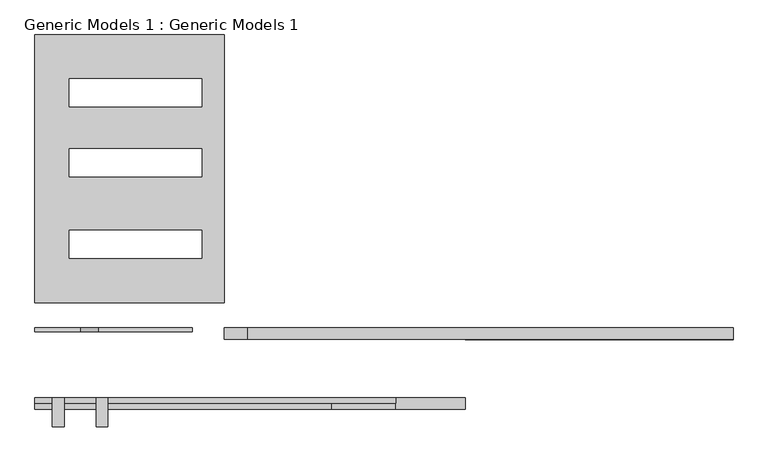
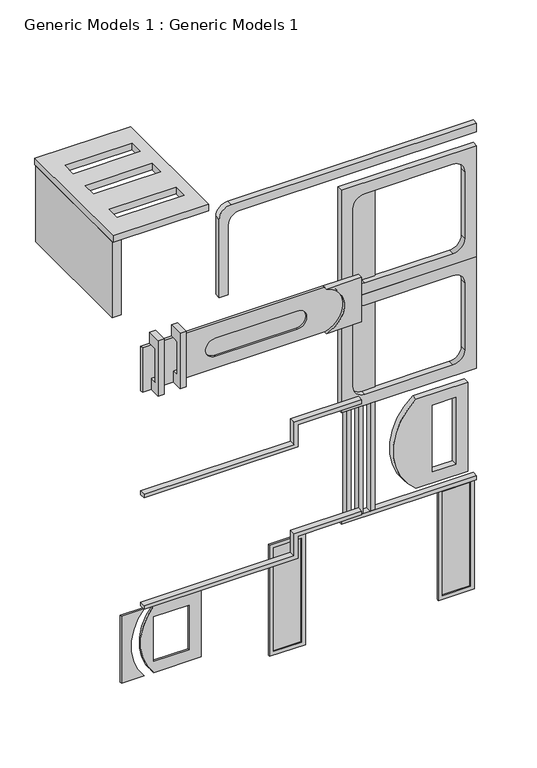
"""IFC4 building model written with IfcOpenShell, lengths in millimetres: proxy geometry, Generic Models 1 : Generic Models 1."""

from ifc_helpers import new_model, si_unit, point, frame, frame_2d, origin, place, context, project, spatial, polyline, circle_curve, trimmed, segment, composite_curve, outline, extrude, source, transform, mapped, element, save
from ifc_brep_helpers import plane_surface, cylinder_surface, revolved_surface, advanced_brep


def generic_models_1_generic_models_1_57c6c2c0(model_context):
    return source(origin(), model_context, "Body", "SolidModel", [
        extrude(outline(polyline([(-720.2794792, -4643.1834702), (-1449.86646, -4643.1834702), (-1449.86646, -4617.7834702), (-720.2794792, -4617.7834702), (-720.2794792, -4643.1834702)])), frame((0.0, 0.0, 101.6), z_axis=(0.0, 0.0, 1.0), x_axis=(1.0, 0.0, 0.0)), (0.0, 0.0, 1.0), 2844.8),
        extrude(outline(polyline([(3655.53354, -4643.1834702), (2925.9465593, -4643.1834702), (2925.9465593, -4617.7834702), (3655.53354, -4617.7834702), (3655.53354, -4643.1834702)])), frame((0.0, 0.0, 101.6), z_axis=(0.0, 0.0, 1.0), x_axis=(1.0, 0.0, 0.0)), (0.0, 0.0, 1.0), 2844.8),
        extrude(outline(polyline([(-5386.86646, -4287.5834702), (-5386.86646, -782.3834702), (-2910.36646, -782.3834702), (-2910.36646, -4287.5834702), (-5386.86646, -4287.5834702)]), holes=[polyline([(-4939.2066105, -1357.9744879), (-4939.2066105, -1726.342691), (-3202.46646, -1726.342691), (-3202.46646, -1357.9744879), (-4939.2066105, -1357.9744879)]), polyline([(-4939.2066105, -2272.3744879), (-4939.2066105, -2640.742691), (-3202.46646, -2640.742691), (-3202.46646, -2272.3744879), (-4939.2066105, -2272.3744879)]), polyline([(-4939.2066105, -3339.1744879), (-4939.2066105, -3707.542691), (-3202.46646, -3707.542691), (-3202.46646, -3339.1744879), (-4939.2066105, -3339.1744879)])]), frame((0.0, 0.0, 12446.0), z_axis=(0.0, 0.0, 1.0), x_axis=(1.0, 0.0, 0.0)), (0.0, 0.0, 1.0), 177.8),
        extrude(outline(polyline([(-5158.26646, -828.55737), (-5158.26646, -4250.1400698), (-5386.86646, -4250.1400698), (-5386.86646, -828.55737), (-5158.26646, -828.55737)])), frame((0.0, 0.0, 10363.2), z_axis=(0.0, 0.0, 1.0), x_axis=(1.0, 0.0, 0.0)), (0.0, 0.0, 1.0), 2082.8),
        extrude(outline(polyline([(3048.0, -618.6794792), (3048.0, -1551.46646), (0.0, -1551.46646), (0.0, -618.6794792), (3048.0, -618.6794792)]), holes=[polyline([(2946.4, -1449.86646), (2946.4, -720.2794792), (101.6, -720.2794792), (101.6, -1449.86646), (2946.4, -1449.86646)])]), frame((0.0, -4668.5834702, 0.0), z_axis=(0.0, 1.0, 0.0), x_axis=(0.0, 0.0, 1.0)), (0.0, 0.0, 1.0), 50.8),
        extrude(outline(polyline([(3048.0, 3757.13354), (3048.0, 2824.3465593), (0.0, 2824.3465593), (0.0, 3757.13354), (3048.0, 3757.13354)]), holes=[polyline([(2946.4, 2925.9465593), (2946.4, 3655.53354), (101.6, 3655.53354), (101.6, 2925.9465593), (2946.4, 2925.9465593)])]), frame((0.0, -4668.5834702, 0.0), z_axis=(0.0, 1.0, 0.0), x_axis=(0.0, 0.0, 1.0)), (0.0, 0.0, 1.0), 50.8),
        extrude(outline(composite_curve([segment(trimmed(circle_curve(frame_2d((1524.0, -3759.0385027)), 1382.6677375), [point((609.6, -4796.1704674))], [point((2438.4, -4796.1704674))], True, "CARTESIAN"), True, "CONTINUOUS"), segment(polyline([(2438.4, -4796.1704674), (2438.4, -5386.86646), (609.6, -5386.86646), (609.6, -4796.1704674)]), True, "CONTINUOUS")], self_intersect=False)), frame((0.0, -4668.5834702, 0.0), z_axis=(0.0, 1.0, 0.0), x_axis=(0.0, 0.0, 1.0)), (0.0, 0.0, 1.0), 50.8),
        extrude(outline(composite_curve([segment(polyline([(2438.4, -3329.46646), (2438.4, -4548.66646)]), True, "CONTINUOUS"), segment(trimmed(circle_curve(frame_2d((1524.0, -3511.5344952)), 1382.6677375), [point((2438.4, -4548.66646))], [point((609.6, -4548.66646))], False, "CARTESIAN"), True, "CONTINUOUS"), segment(polyline([(609.6, -4548.66646), (609.6, -3329.46646), (2438.4, -3329.46646)]), True, "CONTINUOUS")], self_intersect=False), holes=[polyline([(2133.6, -3634.26646), (914.4, -3634.26646), (914.4, -4548.66646), (2133.6, -4548.66646), (2133.6, -3634.26646)])]), frame((0.0, -4668.5834702, 0.0), z_axis=(0.0, 1.0, 0.0), x_axis=(0.0, 0.0, 1.0)), (0.0, 0.0, 1.0), 50.8),
        advanced_brep(
        [(-662.46646, -5608.3834702, 9144.0), (-662.46646, -5608.3834702, 10363.2), (-5386.86646, -5608.3834702, 10363.2), (-5386.86646, -5608.3834702, 9144.0), (-1373.66646, -5608.3834702, 9962.3227004), (-1373.66646, -5608.3834702, 9467.7949612), (-3496.9351426, -5608.3834702, 9467.7949612), (-3496.9351426, -5608.3834702, 9962.3227004), (-662.46646, -5532.1834702, 9144.0), (-5386.86646, -5532.1834702, 9144.0), (-5386.86646, -5532.1834702, 10363.2), (-662.46646, -5532.1834702, 10363.2), (-1373.66646, -5557.5834702, 9962.3227004), (-3496.9351426, -5557.5834702, 9962.3227004), (-3496.9351426, -5557.5834702, 9467.7949612), (-1373.66646, -5557.5834702, 9467.7949612)],
        [
            (0, 1, circle_curve(frame((-823.3880759, -5608.3834702, 9753.6), z_axis=(0.0, -1.0, 0.0), x_axis=(1.0, 0.0, 0.0)), 630.4822967)),
            (1, 2),
            (2, 3),
            (3, 0),
            (4, 5, circle_curve(frame((-1373.66646, -5608.3834702, 9715.0588308), z_axis=(0.0, 1.0, 0.0), x_axis=(-1.0, 0.0, 0.0)), 247.2638696)),
            (5, 6),
            (6, 7, circle_curve(frame((-3496.9351426, -5608.3834702, 9715.0588308), z_axis=(0.0, 1.0, 0.0), x_axis=(-1.0, 0.0, 0.0)), 247.2638696)),
            (7, 4),
            (8, 9),
            (9, 10),
            (10, 11),
            (11, 8, circle_curve(frame((-823.3880759, -5532.1834702, 9753.6), z_axis=(0.0, 1.0, 0.0), x_axis=(1.0, 0.0, 0.0)), 630.4822967)),
            (0, 8),
            (11, 1),
            (10, 2),
            (9, 3),
            (12, 13),
            (13, 14, circle_curve(frame((-3496.9351426, -5557.5834702, 9715.0588308), z_axis=(0.0, -1.0, 0.0), x_axis=(-1.0, 0.0, 0.0)), 247.2638696)),
            (14, 15),
            (15, 12, circle_curve(frame((-1373.66646, -5557.5834702, 9715.0588308), z_axis=(0.0, -1.0, 0.0), x_axis=(-1.0, 0.0, 0.0)), 247.2638696)),
            (15, 5),
            (4, 12),
            (14, 6),
            (13, 7),
        ],
        [
            plane_surface(frame((-192.9057792, -5608.3834702, 9753.6), z_axis=(0.0, -1.0, 0.0), x_axis=(0.0, 0.0, 1.0))),
            plane_surface(frame((-192.9057792, -5532.1834702, 9753.6), z_axis=(0.0, 1.0, 0.0), x_axis=(0.0, 0.0, -1.0))),
            cylinder_surface(frame((-823.3880759, -5532.1834702, 9753.6), z_axis=(0.0, -1.0, 0.0), x_axis=(1.0, 0.0, 0.0)), 630.4822967),
            plane_surface(frame((-662.46646, -5608.3834702, 10363.2), z_axis=(0.0, 0.0, 1.0), x_axis=(0.0, 1.0, 0.0))),
            plane_surface(frame((-5386.86646, -5608.3834702, 10363.2), z_axis=(-1.0, 0.0, 0.0), x_axis=(0.0, 1.0, 0.0))),
            plane_surface(frame((-5386.86646, -5608.3834702, 9144.0), z_axis=(0.0, 0.0, -1.0), x_axis=(0.0, 1.0, 0.0))),
            plane_surface(frame((-1620.9303296, -5557.5834702, 9715.0588308), z_axis=(0.0, -1.0, 0.0), x_axis=(0.0, 0.0, 1.0))),
            revolved_surface(polyline([(-1620.9303295999998, -5557.5834702, 9715.0588308), (-1620.9303295999998, -5608.3834702, 9715.0588308)]), (-1373.66646, -5608.3834702, 9715.0588308), (0.0, 1.0, 0.0)),
            plane_surface(frame((-1373.66646, -5557.5834702, 9467.7949612), z_axis=(0.0, 0.0, 1.0), x_axis=(0.0, -1.0, 0.0))),
            revolved_surface(polyline([(-3744.1990121999997, -5557.5834702, 9715.0588308), (-3744.1990121999997, -5608.3834702, 9715.0588308)]), (-3496.9351426, -5608.3834702, 9715.0588308), (0.0, 1.0, 0.0)),
            plane_surface(frame((-3496.9351426, -5557.5834702, 9962.3227004), z_axis=(0.0, 0.0, -1.0), x_axis=(0.0, -1.0, 0.0))),
        ],
        [
            (0, [[1, 2, 3, 4], [5, 6, 7, 8]]),
            (1, [[9, 10, 11, 12]]),
            (2, [[-1, 13, -12, 14]]),
            (3, [[-2, -14, -11, 15]]),
            (4, [[-3, -15, -10, 16]]),
            (5, [[-4, -16, -9, -13]]),
            (6, [[17, 18, 19, 20]]),
            (7, [[-20, 21, -5, 22]]),
            (8, [[-19, 23, -6, -21]]),
            (9, [[-18, 24, -7, -23]]),
            (10, [[-17, -22, -8, -24]]),
        ],
    ),
        extrude(outline(polyline([(-5532.1834702, 10668.0), (-5532.1834702, 10363.2), (-5684.5834702, 10363.2), (-5786.1834702, 10363.2), (-5786.1834702, 9448.8), (-5532.1834702, 9448.8), (-5532.1834702, 9144.0), (-5913.1834702, 9144.0), (-5913.1834702, 10668.0), (-5532.1834702, 10668.0)])), frame((-5158.26646, 0.0, 0.0), z_axis=(1.0, 0.0, 0.0), x_axis=(0.0, 1.0, 0.0)), (0.0, 0.0, 1.0), 152.4),
        extrude(outline(polyline([(-5532.1834702, 10668.0), (-5532.1834702, 10363.2), (-5684.5834702, 10363.2), (-5786.1834702, 10363.2), (-5786.1834702, 9448.8), (-5532.1834702, 9448.8), (-5532.1834702, 9144.0), (-5913.1834702, 9144.0), (-5913.1834702, 10668.0), (-5532.1834702, 10668.0)])), frame((-4586.76646, 0.0, 0.0), z_axis=(1.0, 0.0, 0.0), x_axis=(0.0, 1.0, 0.0)), (0.0, 0.0, 1.0), 152.4),
        extrude(outline(composite_curve([segment(trimmed(circle_curve(frame_2d((12496.8, -2605.56646)), 304.8), [point((12801.6, -2605.56646))], [point((12496.8, -2910.36646))], False, "CARTESIAN"), True, "CONTINUOUS"), segment(polyline([(12496.8, -2910.36646), (10363.2, -2910.36646), (10363.2, -2681.76646), (12268.2, -2681.76646)]), True, "CONTINUOUS"), segment(trimmed(circle_curve(frame_2d((12268.2, -2376.96646)), 304.8), [point((12268.2, -2681.76646))], [point((12573.0, -2376.96646))], True, "CARTESIAN"), True, "CONTINUOUS"), segment(polyline([(12573.0, -2376.96646), (12573.0, 3757.13354), (12801.6, 3757.13354), (12801.6, -2605.56646)]), True, "CONTINUOUS")], self_intersect=False)), frame((0.0, -4770.1834702, 0.0), z_axis=(0.0, 1.0, 0.0), x_axis=(0.0, 0.0, 1.0)), (0.0, 0.0, 1.0), 152.4),
        extrude(outline(composite_curve([segment(polyline([(9144.0, 251.93354), (10363.2, 251.93354), (10363.2, -662.46646)]), True, "CONTINUOUS"), segment(trimmed(circle_curve(frame_2d((9753.6, -823.3880759)), 630.4822967), [point((10363.2, -662.46646))], [point((9144.0, -662.46646))], True, "CARTESIAN"), True, "CONTINUOUS"), segment(polyline([(9144.0, -662.46646), (9144.0, 251.93354)]), True, "CONTINUOUS")], self_intersect=False)), frame((0.0, -5684.5834702, 0.0), z_axis=(0.0, 1.0, 0.0), x_axis=(0.0, 0.0, 1.0)), (0.0, 0.0, 1.0), 152.4),
        extrude(outline(polyline([(7010.4, -1500.66646), (6400.8, -1500.66646), (6400.8, -5386.86646), (6299.2, -5386.86646), (6299.2, -1399.06646), (6908.8, -1399.06646), (6908.8, 251.93354), (7010.4, 251.93354), (7010.4, -1500.66646)])), frame((0.0, -5684.5834702, 0.0), z_axis=(0.0, 1.0, 0.0), x_axis=(0.0, 0.0, 1.0)), (0.0, 0.0, 1.0), 152.4),
        extrude(outline(polyline([(3962.4, -1500.66646), (3352.8, -1500.66646), (3352.8, -5386.86646), (3251.2, -5386.86646), (3251.2, -1399.06646), (3860.8, -1399.06646), (3860.8, 251.93354), (3962.4, 251.93354), (3962.4, -1500.66646)])), frame((0.0, -5684.5834702, 0.0), z_axis=(0.0, 1.0, 0.0), x_axis=(0.0, 0.0, 1.0)), (0.0, 0.0, 1.0), 152.4),
        extrude(outline(polyline([(505.7599653, -4617.7834702), (505.7599653, -4770.1834702), (385.7579468, -4770.1834702), (385.7579468, -4617.7834702), (505.7599653, -4617.7834702)])), frame((0.0, 0.0, 3149.6), z_axis=(0.0, 0.0, 1.0), x_axis=(1.0, 0.0, 0.0)), (0.0, 0.0, 1.0), 2946.4),
        extrude(outline(polyline([(816.9099653, -4617.7834702), (816.9099653, -4770.1834702), (696.9079468, -4770.1834702), (696.9079468, -4617.7834702), (816.9099653, -4617.7834702)])), frame((0.0, 0.0, 3149.6), z_axis=(0.0, 0.0, 1.0), x_axis=(1.0, 0.0, 0.0)), (0.0, 0.0, 1.0), 2946.4),
        extrude(outline(polyline([(1121.7099653, -4617.7834702), (1121.7099653, -4770.1834702), (1001.7079468, -4770.1834702), (1001.7079468, -4617.7834702), (1121.7099653, -4617.7834702)])), frame((0.0, 0.0, 3149.6), z_axis=(0.0, 0.0, 1.0), x_axis=(1.0, 0.0, 0.0)), (0.0, 0.0, 1.0), 2946.4),
        extrude(outline(polyline([(3757.13354, -4770.1834702), (251.93354, -4770.1834702), (251.93354, -4617.7834702), (3757.13354, -4617.7834702), (3757.13354, -4770.1834702)])), frame((0.0, 0.0, 3048.0), z_axis=(0.0, 0.0, 1.0), x_axis=(1.0, 0.0, 0.0)), (0.0, 0.0, 1.0), 101.6),
        extrude(outline(composite_curve([segment(polyline([(5791.2, 3528.53354), (5791.2, 2191.4893246)]), True, "CONTINUOUS"), segment(trimmed(circle_curve(frame_2d((4572.0, 3127.4063803)), 1537.0066282), [point((5791.2, 2191.4893246))], [point((3352.8, 2191.4893246))], False, "CARTESIAN"), True, "CONTINUOUS"), segment(polyline([(3352.8, 2191.4893246), (3352.8, 3528.53354), (5791.2, 3528.53354)]), True, "CONTINUOUS")], self_intersect=False), holes=[polyline([(5486.4, 3223.73354), (3657.6, 3223.73354), (3657.6, 2614.13354), (5486.4, 2614.13354), (5486.4, 3223.73354)])]), frame((0.0, -4770.1834702, 0.0), z_axis=(0.0, 1.0, 0.0), x_axis=(0.0, 0.0, 1.0)), (0.0, 0.0, 1.0), 152.4),
        extrude(outline(composite_curve([segment(polyline([(9448.8, 1200.1844706), (11887.2, 1200.1844706), (11887.2, 861.53354)]), True, "CONTINUOUS"), segment(trimmed(circle_curve(frame_2d((11582.4, 861.53354)), 304.8), [point((11887.2, 861.53354))], [point((11582.4, 556.73354))], False, "CARTESIAN"), True, "CONTINUOUS"), segment(polyline([(11582.4, 556.73354), (9753.6, 556.73354)]), True, "CONTINUOUS"), segment(trimmed(circle_curve(frame_2d((9753.6, 861.53354)), 304.8), [point((9753.6, 556.73354))], [point((9448.8, 861.53354))], False, "CARTESIAN"), True, "CONTINUOUS"), segment(polyline([(9448.8, 861.53354), (9448.8, 1200.1844706)]), True, "CONTINUOUS")], self_intersect=False)), frame((0.0, -4643.1834702, 0.0), z_axis=(0.0, 1.0, 0.0), x_axis=(0.0, 0.0, 1.0)), (0.0, 0.0, 1.0), 25.4),
        extrude(outline(composite_curve([segment(polyline([(6400.8, 1200.1844706), (8839.2, 1200.1844706), (8839.2, 861.53354)]), True, "CONTINUOUS"), segment(trimmed(circle_curve(frame_2d((8534.4, 861.53354)), 304.8), [point((8839.2, 861.53354))], [point((8534.4, 556.73354))], False, "CARTESIAN"), True, "CONTINUOUS"), segment(polyline([(8534.4, 556.73354), (6705.6, 556.73354)]), True, "CONTINUOUS"), segment(trimmed(circle_curve(frame_2d((6705.6, 861.53354)), 304.8), [point((6705.6, 556.73354))], [point((6400.8, 861.53354))], False, "CARTESIAN"), True, "CONTINUOUS"), segment(polyline([(6400.8, 861.53354), (6400.8, 1200.1844706)]), True, "CONTINUOUS")], self_intersect=False)), frame((0.0, -4643.1834702, 0.0), z_axis=(0.0, 1.0, 0.0), x_axis=(0.0, 0.0, 1.0)), (0.0, 0.0, 1.0), 25.4),
        extrude(outline(polyline([(9144.0, 251.93354), (6096.0, 251.93354), (6096.0, 3757.13354), (9144.0, 3757.13354), (9144.0, 251.93354)]), holes=[composite_curve([segment(polyline([(8839.2, 861.53354), (8839.2, 3147.53354)]), True, "CONTINUOUS"), segment(trimmed(circle_curve(frame_2d((8534.4, 3147.53354)), 304.8), [point((8839.2, 3147.53354))], [point((8534.4, 3452.33354))], True, "CARTESIAN"), True, "CONTINUOUS"), segment(polyline([(8534.4, 3452.33354), (6705.6, 3452.33354)]), True, "CONTINUOUS"), segment(trimmed(circle_curve(frame_2d((6705.6, 3147.53354)), 304.8), [point((6705.6, 3452.33354))], [point((6400.8, 3147.53354))], True, "CARTESIAN"), True, "CONTINUOUS"), segment(polyline([(6400.8, 3147.53354), (6400.8, 861.53354)]), True, "CONTINUOUS"), segment(trimmed(circle_curve(frame_2d((6705.6, 861.53354)), 304.8), [point((6400.8, 861.53354))], [point((6705.6, 556.73354))], True, "CARTESIAN"), True, "CONTINUOUS"), segment(polyline([(6705.6, 556.73354), (8534.4, 556.73354)]), True, "CONTINUOUS"), segment(trimmed(circle_curve(frame_2d((8534.4, 861.53354)), 304.8), [point((8534.4, 556.73354))], [point((8839.2, 861.53354))], True, "CARTESIAN"), True, "CONTINUOUS")], self_intersect=False)]), frame((0.0, -4770.1834702, 0.0), z_axis=(0.0, 1.0, 0.0), x_axis=(0.0, 0.0, 1.0)), (0.0, 0.0, 1.0), 152.4),
        extrude(outline(polyline([(12192.0, 251.93354), (9144.0, 251.93354), (9144.0, 3757.13354), (12192.0, 3757.13354), (12192.0, 251.93354)]), holes=[composite_curve([segment(polyline([(11887.2, 861.53354), (11887.2, 3147.53354)]), True, "CONTINUOUS"), segment(trimmed(circle_curve(frame_2d((11582.4, 3147.53354)), 304.8), [point((11887.2, 3147.53354))], [point((11582.4, 3452.33354))], True, "CARTESIAN"), True, "CONTINUOUS"), segment(polyline([(11582.4, 3452.33354), (9753.6, 3452.33354)]), True, "CONTINUOUS"), segment(trimmed(circle_curve(frame_2d((9753.6, 3147.53354)), 304.8), [point((9753.6, 3452.33354))], [point((9448.8, 3147.53354))], True, "CARTESIAN"), True, "CONTINUOUS"), segment(polyline([(9448.8, 3147.53354), (9448.8, 861.53354)]), True, "CONTINUOUS"), segment(trimmed(circle_curve(frame_2d((9753.6, 861.53354)), 304.8), [point((9448.8, 861.53354))], [point((9753.6, 556.73354))], True, "CARTESIAN"), True, "CONTINUOUS"), segment(polyline([(9753.6, 556.73354), (11582.4, 556.73354)]), True, "CONTINUOUS"), segment(trimmed(circle_curve(frame_2d((11582.4, 861.53354)), 304.8), [point((11582.4, 556.73354))], [point((11887.2, 861.53354))], True, "CARTESIAN"), True, "CONTINUOUS")], self_intersect=False)]), frame((0.0, -4770.1834702, 0.0), z_axis=(0.0, 1.0, 0.0), x_axis=(0.0, 0.0, 1.0)), (0.0, 0.0, 1.0), 152.4),
    ])


if __name__ == "__main__":
    model = new_model("IFC4")
    model_context = context("Model", 3, world=origin())
    ifc_project = project(units=[si_unit("LENGTHUNIT", "METRE", prefix="MILLI")], contexts=[model_context])
    site = spatial("IfcSite", under=ifc_project)
    building = spatial("IfcBuilding", under=site)
    placement = place(None, origin())
    generic_models_1_generic_models_1_shape = generic_models_1_generic_models_1_57c6c2c0(model_context)
    element("IfcBuildingElementProxy", 1, Name="Generic Models 1 : Generic Models 1", ObjectType="Generic Models 1 : Generic Models 1", at=placement, inside=building, context=model_context, shape_type="MappedRepresentation", body=[
        mapped(generic_models_1_generic_models_1_shape, transform((0.0, 0.0, 0.0), x_axis=(1.0, 0.0, 0.0), y_axis=(0.0, 1.0, 0.0), z_axis=(0.0, 0.0, 1.0))),
    ])
    save(model, "model.ifc")

# Revit data of these elements
# Element 1 (IfcBuildingElementProxy, "Generic Models 1 : Generic Models 1")
#   Materials on its faces: "03 white", "02 colour", "04 tiles", "01 colour"
# Materials
#   "03 white": class "Generic", colour RGB 120 120 120, transparency 0, Cost = 0
#   "02 colour": class "Generic", colour RGB 120 120 120, transparency 0, Cost = 0
#   "04 tiles": class "Generic", colour RGB 120 120 120, transparency 0, Cost = 0
#   "01 colour": class "Generic", colour RGB 120 120 120, transparency 0, Cost = 0
